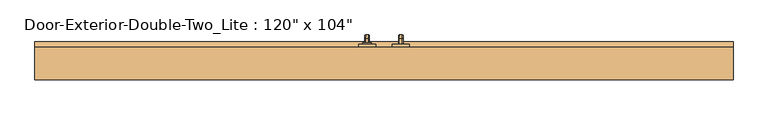
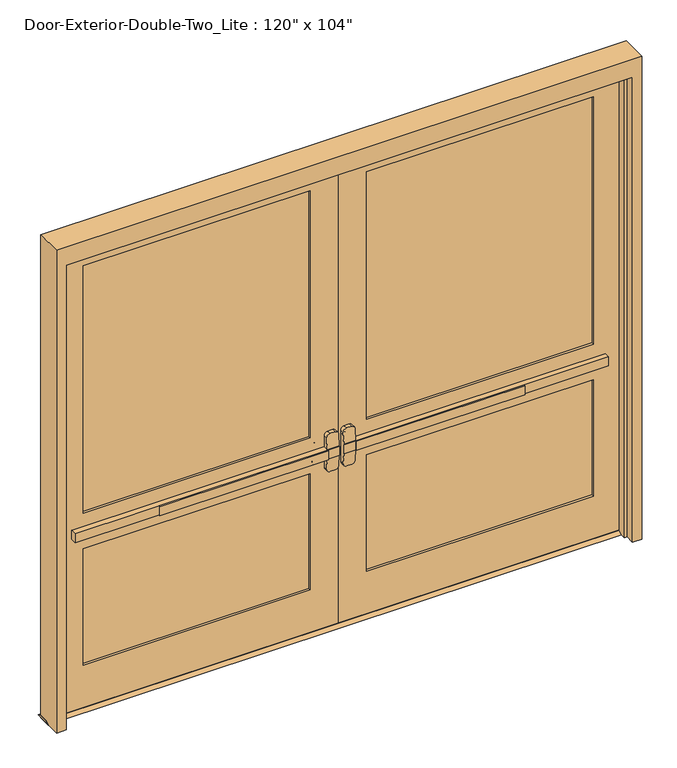
"""IFC4 building model written with IfcOpenShell, lengths in millimetres: door geometry."""

from ifc_helpers import new_model, si_unit, point, frame, frame_2d, origin, place, context, project, spatial, polyline, circle_curve, ellipse_curve, trimmed, segment, composite_curve, outline, extrude, faceted_brep, source, transform, mapped, element, save
from ifc_brep_helpers import plane_surface, cylinder_surface, revolved_surface, advanced_brep


def door_7b75190e(model_context):
    return source(origin(), model_context, "Body", "SolidModel", [
        extrude(outline(polyline([(-982.1333333, 0.0), (-982.1333333, 6.35), (-76.2, 6.35), (-76.2, 0.0), (-982.1333333, 0.0)])), frame((0.0, 0.0, 990.6), z_axis=(0.0, 0.0, 1.0), x_axis=(1.0, 0.0, 0.0)), (0.0, 0.0, 1.0), 50.8),
        advanced_brep(
        [(-12.7, 6.35, 1041.4), (-76.2, 6.35, 1041.4), (-1435.1, 6.35, 1041.4), (-1435.1, 6.35, 990.6), (-76.2, 6.35, 990.6), (-12.7, 6.35, 990.6), (-1435.1, 38.1, 1041.4), (-76.2, 38.1, 1041.4), (-76.2, 38.1, 1104.9), (-57.15, 38.1, 1123.95), (-31.75, 38.1, 1123.95), (-12.7, 38.1, 1104.9), (-12.7, 38.1, 927.1), (-31.75, 38.1, 908.05), (-57.15, 38.1, 908.05), (-76.2, 38.1, 927.1), (-76.2, 38.1, 990.6), (-1435.1, 38.1, 990.6), (-12.7, 9.5252467, 1041.4), (-76.2, 9.5252467, 1041.4), (-12.7, 9.5252467, 990.6), (-12.7, 14.5354269, 927.1), (-12.7, 14.5354269, 1104.9), (-76.2, 9.5252467, 990.6), (-76.2, 14.5354269, 1104.9), (-76.2, 14.5354269, 927.1), (-57.15, 16.038481, 1123.95), (-31.75, 16.038481, 1123.95), (-31.75, 16.038481, 908.05), (-57.15, 16.038481, 908.05)],
        [
            (0, 1),
            (1, 2),
            (2, 3),
            (3, 4),
            (4, 5),
            (5, 0),
            (6, 7),
            (7, 8),
            (8, 9, circle_curve(frame((-57.15, 38.1, 1104.9), z_axis=(0.0, 1.0, 0.0), x_axis=(-1.0, 0.0, 0.0)), 19.05)),
            (9, 10),
            (10, 11, circle_curve(frame((-31.75, 38.1, 1104.9), z_axis=(0.0, 1.0, 0.0), x_axis=(-1.0, 0.0, 0.0)), 19.05)),
            (11, 12),
            (12, 13, circle_curve(frame((-31.75, 38.1, 927.1), z_axis=(0.0, 1.0, 0.0), x_axis=(-1.0, 0.0, 0.0)), 19.05)),
            (13, 14),
            (14, 15, circle_curve(frame((-57.15, 38.1, 927.1), z_axis=(0.0, 1.0, 0.0), x_axis=(-1.0, 0.0, 0.0)), 19.05)),
            (15, 16),
            (16, 17),
            (17, 6),
            (0, 18),
            (18, 19),
            (19, 7),
            (6, 2),
            (5, 20),
            (20, 21),
            (21, 12),
            (11, 22),
            (22, 18),
            (16, 23),
            (23, 20),
            (3, 17),
            (19, 24),
            (24, 8),
            (15, 25),
            (25, 23),
            (9, 26),
            (26, 27),
            (27, 10),
            (13, 28),
            (28, 29),
            (29, 14),
            (29, 25, ellipse_curve(frame((-57.15, 14.5354269, 927.1), z_axis=(0.0, 0.9969018152893365, 0.07865602756830282), x_axis=(0.0, -0.07865602756830208, 0.9969018152893365)), 19.1092038, 19.05)),
            (24, 26, ellipse_curve(frame((-57.15, 14.5354269, 1104.9), z_axis=(0.0, 0.9969018152893376, -0.07865602756828934), x_axis=(0.0, -0.078656027568288, -0.9969018152893377)), 19.1092038, 19.05)),
            (27, 22, ellipse_curve(frame((-31.75, 14.5354269, 1104.9), z_axis=(0.0, 0.9969018152893376, -0.07865602756828934), x_axis=(0.0, -0.078656027568288, -0.9969018152893377)), 19.1092038, 19.05)),
            (21, 28, ellipse_curve(frame((-31.75, 14.5354269, 927.1), z_axis=(0.0, 0.9969018152893365, 0.07865602756830282), x_axis=(0.0, -0.07865602756830208, 0.9969018152893365)), 19.1092038, 19.05)),
        ],
        [
            plane_surface(frame((-12.7, 6.35, 1041.4), z_axis=(0.0, -1.0, 0.0), x_axis=(1.0, 0.0, 0.0))),
            plane_surface(frame((-12.7, 38.1, 1041.4), z_axis=(0.0, 1.0, 0.0), x_axis=(-1.0, 0.0, 0.0))),
            plane_surface(frame((-1435.1, 6.35, 1041.4), z_axis=(0.0, 0.0, 1.0), x_axis=(0.0, 1.0, 0.0))),
            plane_surface(frame((-12.7, 6.35, 1041.4), z_axis=(1.0, 0.0, 0.0), x_axis=(0.0, 1.0, 0.0))),
            plane_surface(frame((-12.7, 6.35, 990.6), z_axis=(0.0, 0.0, -1.0), x_axis=(0.0, 1.0, 0.0))),
            plane_surface(frame((-1435.1, 6.35, 990.6), z_axis=(-1.0, 0.0, 0.0), x_axis=(0.0, 1.0, 0.0))),
            plane_surface(frame((-76.2, 9.5252467, 927.1), z_axis=(-1.0, 0.0, 0.0), x_axis=(0.0, 1.0, 0.0))),
            plane_surface(frame((-57.15, 9.5252467, 1123.95), z_axis=(0.0, 0.0, 1.0), x_axis=(0.0, 1.0, 0.0))),
            plane_surface(frame((-31.75, 9.5252467, 908.05), z_axis=(0.0, 0.0, -1.0), x_axis=(0.0, 1.0, 0.0))),
            cylinder_surface(frame((-57.15, 38.1, 927.1), z_axis=(0.0, -1.0, 0.0), x_axis=(-1.0, 0.0, 0.0)), 19.05),
            cylinder_surface(frame((-57.15, 38.1, 1104.9), z_axis=(0.0, -1.0, 0.0), x_axis=(-1.0, 0.0, 0.0)), 19.05),
            cylinder_surface(frame((-31.75, 38.1, 1104.9), z_axis=(0.0, -1.0, 0.0), x_axis=(-1.0, 0.0, 0.0)), 19.05),
            cylinder_surface(frame((-31.75, 38.1, 927.1), z_axis=(0.0, -1.0, 0.0), x_axis=(-1.0, 0.0, 0.0)), 19.05),
            plane_surface(frame((-76.2, 9.5252467, 1041.4), z_axis=(0.0, -0.9969018152893376, 0.07865602756828934), x_axis=(1.0, 0.0, 0.0))),
            plane_surface(frame((-76.2, 16.038481, 908.05), z_axis=(0.0, -0.9969018152893365, -0.07865602756830282), x_axis=(1.0, 0.0, 0.0))),
        ],
        [
            (0, [[1, 2, 3, 4, 5, 6]]),
            (1, [[7, 8, 9, 10, 11, 12, 13, 14, 15, 16, 17, 18]]),
            (2, [[-2, -1, 19, 20, 21, -7, 22]]),
            (3, [[23, 24, 25, -12, 26, 27, -19, -6]]),
            (4, [[-17, 28, 29, -23, -5, -4, 30]]),
            (5, [[-22, -18, -30, -3]]),
            (6, [[-21, 31, 32, -8]]),
            (6, [[33, 34, -28, -16]]),
            (7, [[35, 36, 37, -10]]),
            (8, [[38, 39, 40, -14]]),
            (9, [[-40, 41, -33, -15]]),
            (10, [[-32, 42, -35, -9]]),
            (11, [[-37, 43, -26, -11]]),
            (12, [[-25, 44, -38, -13]]),
            (13, [[-27, -43, -36, -42, -31, -20]]),
            (14, [[-29, -34, -41, -39, -44, -24]]),
        ],
    ),
        extrude(outline(polyline([(82.55, 12.7), (107.95, 0.0), (12.7, 0.0), (38.1, 12.7), (82.55, 12.7)])), frame((-1574.8, 0.0, 0.0), z_axis=(1.0, 0.0, 0.0), x_axis=(0.0, 1.0, 0.0)), (0.0, 0.0, 1.0), 3149.6),
        extrude(outline(polyline([(982.1333333, 0.0), (76.2, 0.0), (76.2, 6.35), (982.1333333, 6.35), (982.1333333, 0.0)])), frame((0.0, 0.0, 990.6), z_axis=(0.0, 0.0, 1.0), x_axis=(1.0, 0.0, 0.0)), (0.0, 0.0, 1.0), 50.8),
        advanced_brep(
        [(12.7, 6.35, 1041.4), (12.7, 6.35, 990.6), (76.2, 6.35, 990.6), (1435.1, 6.35, 990.6), (1435.1, 6.35, 1041.4), (76.2, 6.35, 1041.4), (1435.1, 38.1, 1041.4), (1435.1, 38.1, 990.6), (76.2, 38.1, 990.6), (76.2, 38.1, 927.1), (57.15, 38.1, 908.05), (31.75, 38.1, 908.05), (12.7, 38.1, 927.1), (12.7, 38.1, 1104.9), (31.75, 38.1, 1123.95), (57.15, 38.1, 1123.95), (76.2, 38.1, 1104.9), (76.2, 38.1, 1041.4), (76.2, 9.5252467, 1041.4), (12.7, 9.5252467, 1041.4), (12.7, 14.5354269, 1104.9), (12.7, 14.5354269, 927.1), (12.7, 9.5252467, 990.6), (76.2, 9.5252467, 990.6), (76.2, 14.5354269, 927.1), (76.2, 14.5354269, 1104.9), (31.75, 16.038481, 1123.95), (57.15, 16.038481, 1123.95), (57.15, 16.038481, 908.05), (31.75, 16.038481, 908.05)],
        [
            (0, 1),
            (1, 2),
            (2, 3),
            (3, 4),
            (4, 5),
            (5, 0),
            (6, 7),
            (7, 8),
            (8, 9),
            (9, 10, circle_curve(frame((57.15, 38.1, 927.1), z_axis=(0.0, 1.0, 0.0), x_axis=(1.0, 0.0, 0.0)), 19.05)),
            (10, 11),
            (11, 12, circle_curve(frame((31.75, 38.1, 927.1), z_axis=(0.0, 1.0, 0.0), x_axis=(1.0, 0.0, 0.0)), 19.05)),
            (12, 13),
            (13, 14, circle_curve(frame((31.75, 38.1, 1104.9), z_axis=(0.0, 1.0, 0.0), x_axis=(1.0, 0.0, 0.0)), 19.05)),
            (14, 15),
            (15, 16, circle_curve(frame((57.15, 38.1, 1104.9), z_axis=(0.0, 1.0, 0.0), x_axis=(1.0, 0.0, 0.0)), 19.05)),
            (16, 17),
            (17, 6),
            (4, 6),
            (17, 18),
            (18, 19),
            (19, 0),
            (19, 20),
            (20, 13),
            (12, 21),
            (21, 22),
            (22, 1),
            (7, 3),
            (22, 23),
            (23, 8),
            (23, 24),
            (24, 9),
            (16, 25),
            (25, 18),
            (14, 26),
            (26, 27),
            (27, 15),
            (10, 28),
            (28, 29),
            (29, 11),
            (24, 28, ellipse_curve(frame((57.15, 14.5354269, 927.1), z_axis=(0.0, 0.9969018152893365, 0.07865602756830282), x_axis=(0.0, -0.07865602756830208, 0.9969018152893365)), 19.1092038, 19.05)),
            (27, 25, ellipse_curve(frame((57.15, 14.5354269, 1104.9), z_axis=(0.0, 0.9969018152893376, -0.07865602756828934), x_axis=(0.0, -0.078656027568288, -0.9969018152893377)), 19.1092038, 19.05)),
            (20, 26, ellipse_curve(frame((31.75, 14.5354269, 1104.9), z_axis=(0.0, 0.9969018152893376, -0.07865602756828934), x_axis=(0.0, -0.078656027568288, -0.9969018152893377)), 19.1092038, 19.05)),
            (29, 21, ellipse_curve(frame((31.75, 14.5354269, 927.1), z_axis=(0.0, 0.9969018152893365, 0.07865602756830282), x_axis=(0.0, -0.07865602756830208, 0.9969018152893365)), 19.1092038, 19.05)),
        ],
        [
            plane_surface(frame((12.7, 6.35, 1041.4), z_axis=(0.0, -1.0, 0.0), x_axis=(-1.0, 0.0, 0.0))),
            plane_surface(frame((12.7, 38.1, 1041.4), z_axis=(0.0, 1.0, 0.0), x_axis=(1.0, 0.0, 0.0))),
            plane_surface(frame((1435.1, 6.35, 1041.4), z_axis=(0.0, 0.0, 1.0), x_axis=(0.0, 1.0, 0.0))),
            plane_surface(frame((12.7, 6.35, 1041.4), z_axis=(-1.0, 0.0, 0.0), x_axis=(0.0, 1.0, 0.0))),
            plane_surface(frame((12.7, 6.35, 990.6), z_axis=(0.0, 0.0, -1.0), x_axis=(0.0, 1.0, 0.0))),
            plane_surface(frame((1435.1, 6.35, 990.6), z_axis=(1.0, 0.0, 0.0), x_axis=(0.0, 1.0, 0.0))),
            plane_surface(frame((76.2, 9.5252467, 927.1), z_axis=(1.0, 0.0, 0.0), x_axis=(0.0, 1.0, 0.0))),
            plane_surface(frame((57.15, 9.5252467, 1123.95), z_axis=(0.0, 0.0, 1.0), x_axis=(0.0, 1.0, 0.0))),
            plane_surface(frame((31.75, 9.5252467, 908.05), z_axis=(0.0, 0.0, -1.0), x_axis=(0.0, 1.0, 0.0))),
            cylinder_surface(frame((57.15, 38.1, 927.1), z_axis=(0.0, -1.0, 0.0), x_axis=(1.0, 0.0, 0.0)), 19.05),
            cylinder_surface(frame((57.15, 38.1, 1104.9), z_axis=(0.0, -1.0, 0.0), x_axis=(1.0, 0.0, 0.0)), 19.05),
            cylinder_surface(frame((31.75, 38.1, 1104.9), z_axis=(0.0, -1.0, 0.0), x_axis=(1.0, 0.0, 0.0)), 19.05),
            cylinder_surface(frame((31.75, 38.1, 927.1), z_axis=(0.0, -1.0, 0.0), x_axis=(1.0, 0.0, 0.0)), 19.05),
            plane_surface(frame((76.2, 9.5252467, 1041.4), z_axis=(0.0, -0.9969018152893376, 0.07865602756828934), x_axis=(-1.0, 0.0, 0.0))),
            plane_surface(frame((76.2, 16.038481, 908.05), z_axis=(0.0, -0.9969018152893365, -0.07865602756830282), x_axis=(-1.0, 0.0, 0.0))),
        ],
        [
            (0, [[1, 2, 3, 4, 5, 6]]),
            (1, [[7, 8, 9, 10, 11, 12, 13, 14, 15, 16, 17, 18]]),
            (2, [[19, -18, 20, 21, 22, -6, -5]]),
            (3, [[-1, -22, 23, 24, -13, 25, 26, 27]]),
            (4, [[28, -3, -2, -27, 29, 30, -8]]),
            (5, [[-4, -28, -7, -19]]),
            (6, [[-9, -30, 31, 32]]),
            (6, [[-17, 33, 34, -20]]),
            (7, [[-15, 35, 36, 37]]),
            (8, [[-11, 38, 39, 40]]),
            (9, [[-10, -32, 41, -38]]),
            (10, [[-16, -37, 42, -33]]),
            (11, [[-14, -24, 43, -35]]),
            (12, [[-12, -40, 44, -25]]),
            (13, [[-21, -34, -42, -36, -43, -23]]),
            (14, [[-26, -44, -39, -41, -31, -29]]),
        ],
    ),
        advanced_brep(
        [(66.2, 95.25, 1017.190625), (66.2, 95.25, 1014.809375), (69.771875, 95.25, 1011.2375), (82.6284594, 95.25, 1011.2375), (86.2, 95.25, 1014.8090406), (86.2, 95.25, 1017.190625), (82.628125, 95.25, 1020.7625), (69.771875, 95.25, 1020.7625), (66.2, 95.25, 887.809375), (69.771875, 95.25, 884.2375), (82.628125, 95.25, 884.2375), (86.2, 95.25, 887.809375), (86.2, 95.25, 890.1909594), (82.6284594, 95.25, 893.7625), (69.771875, 95.25, 893.7625), (66.2, 95.25, 890.190625), (66.2, 120.65, 1017.190625), (66.2, 134.540625, 1003.3), (66.2, 134.540625, 901.7), (66.2, 120.65, 887.809375), (66.2, 120.65, 890.190625), (66.2, 132.159375, 901.7), (66.2, 132.159375, 1003.3), (66.2, 120.65, 1014.809375), (69.771875, 120.65, 1011.2375), (82.6284594, 120.65, 1011.2375), (86.2, 120.65, 1014.8090406), (86.2, 132.1590406, 1003.3), (86.2, 132.1590406, 901.7), (86.2, 120.65, 890.1909594), (86.2, 120.65, 887.809375), (86.2, 134.540625, 901.7), (86.2, 134.540625, 1003.3), (86.2, 120.65, 1017.190625), (82.628125, 120.65, 1020.7625), (69.771875, 120.65, 1020.7625), (69.771875, 128.5875, 1003.3), (82.6284594, 128.5875, 1003.3), (82.628125, 138.1125, 1003.3), (69.771875, 138.1125, 1003.3), (69.771875, 128.5875, 901.7), (82.6284594, 128.5875, 901.7), (82.628125, 138.1125, 901.7), (69.771875, 138.1125, 901.7), (69.771875, 120.65, 893.7625), (82.6284594, 120.65, 893.7625), (82.628125, 120.65, 884.2375), (69.771875, 120.65, 884.2375)],
        [
            (0, 1),
            (1, 2, circle_curve(frame((69.771875, 95.25, 1014.809375), z_axis=(0.0, -1.0, 0.0), x_axis=(0.0, 0.0, 1.0)), 3.571875)),
            (2, 3),
            (3, 4, circle_curve(frame((82.6284594, 95.25, 1014.8090406), z_axis=(0.0, -1.0, 0.0), x_axis=(0.0, 0.0, 1.0)), 3.5715406)),
            (4, 5),
            (5, 6, circle_curve(frame((82.628125, 95.25, 1017.190625), z_axis=(0.0, -1.0, 0.0), x_axis=(0.0, 0.0, 1.0)), 3.571875)),
            (6, 7),
            (7, 0, circle_curve(frame((69.771875, 95.25, 1017.190625), z_axis=(0.0, -1.0, 0.0), x_axis=(0.0, 0.0, 1.0)), 3.571875)),
            (8, 9, circle_curve(frame((69.771875, 95.25, 887.809375), z_axis=(0.0, -1.0, 0.0), x_axis=(0.0, 0.0, -1.0)), 3.571875)),
            (9, 10),
            (10, 11, circle_curve(frame((82.628125, 95.25, 887.809375), z_axis=(0.0, -1.0, 0.0), x_axis=(0.0, 0.0, -1.0)), 3.571875)),
            (11, 12),
            (12, 13, circle_curve(frame((82.6284594, 95.25, 890.1909594), z_axis=(0.0, -1.0, 0.0), x_axis=(0.0, 0.0, -1.0)), 3.5715406)),
            (13, 14),
            (14, 15, circle_curve(frame((69.771875, 95.25, 890.190625), z_axis=(0.0, -1.0, 0.0), x_axis=(0.0, 0.0, -1.0)), 3.571875)),
            (15, 8),
            (0, 16),
            (16, 17, circle_curve(frame((66.2, 120.65, 1003.3), z_axis=(-1.0, 0.0, 0.0), x_axis=(0.0, 0.0, 1.0)), 13.890625)),
            (17, 18),
            (18, 19, circle_curve(frame((66.2, 120.65, 901.7), z_axis=(-1.0, 0.0, 0.0), x_axis=(0.0, 1.0, 0.0)), 13.890625)),
            (19, 8),
            (15, 20),
            (20, 21, circle_curve(frame((66.2, 120.65, 901.7), z_axis=(1.0, 0.0, 0.0), x_axis=(0.0, 1.0, 0.0)), 11.509375)),
            (21, 22),
            (22, 23, circle_curve(frame((66.2, 120.65, 1003.3), z_axis=(1.0, 0.0, 0.0), x_axis=(0.0, 0.0, 1.0)), 11.509375)),
            (23, 1),
            (23, 24, circle_curve(frame((69.771875, 120.65, 1014.809375), z_axis=(0.0, -1.0, 0.0), x_axis=(0.0, 0.0, 1.0)), 3.571875)),
            (24, 2),
            (24, 25),
            (25, 3),
            (25, 26, circle_curve(frame((82.6284594, 120.65, 1014.8090406), z_axis=(0.0, -1.0, 0.0), x_axis=(0.0, 0.0, 1.0)), 3.5715406)),
            (26, 4),
            (26, 27, circle_curve(frame((86.2, 120.65, 1003.3), z_axis=(-1.0, 0.0, 0.0), x_axis=(0.0, 0.0, 1.0)), 11.5090406)),
            (27, 28),
            (28, 29, circle_curve(frame((86.2, 120.65, 901.7), z_axis=(-1.0, 0.0, 0.0), x_axis=(0.0, 1.0, 0.0)), 11.5090406)),
            (29, 12),
            (11, 30),
            (30, 31, circle_curve(frame((86.2, 120.65, 901.7), z_axis=(1.0, 0.0, 0.0), x_axis=(0.0, 1.0, 0.0)), 13.890625)),
            (31, 32),
            (32, 33, circle_curve(frame((86.2, 120.65, 1003.3), z_axis=(1.0, 0.0, 0.0), x_axis=(0.0, 0.0, 1.0)), 13.890625)),
            (33, 5),
            (33, 34, circle_curve(frame((82.628125, 120.65, 1017.190625), z_axis=(0.0, -1.0, 0.0), x_axis=(0.0, 0.0, 1.0)), 3.571875)),
            (34, 6),
            (34, 35),
            (35, 7),
            (35, 16, circle_curve(frame((69.771875, 120.65, 1017.190625), z_axis=(0.0, -1.0, 0.0), x_axis=(0.0, 0.0, 1.0)), 3.571875)),
            (36, 24, circle_curve(frame((69.771875, 120.65, 1003.3), z_axis=(1.0, 0.0, 0.0), x_axis=(0.0, 0.0, 1.0)), 7.9375)),
            (22, 36, circle_curve(frame((69.771875, 132.159375, 1003.3), z_axis=(0.0, 0.0, 1.0), x_axis=(0.0, 1.0, 0.0)), 3.571875)),
            (37, 25, circle_curve(frame((82.6284594, 120.65, 1003.3), z_axis=(1.0, 0.0, 0.0), x_axis=(0.0, 0.0, 1.0)), 7.9375)),
            (36, 37),
            (37, 27, circle_curve(frame((82.6284594, 132.1590406, 1003.3), z_axis=(0.0, 0.0, 1.0), x_axis=(0.0, 1.0, 0.0)), 3.5715406)),
            (38, 34, circle_curve(frame((82.628125, 120.65, 1003.3), z_axis=(1.0, 0.0, 0.0), x_axis=(0.0, 0.0, 1.0)), 17.4625)),
            (32, 38, circle_curve(frame((82.628125, 134.540625, 1003.3), z_axis=(0.0, 0.0, 1.0), x_axis=(0.0, 1.0, 0.0)), 3.571875)),
            (39, 35, circle_curve(frame((69.771875, 120.65, 1003.3), z_axis=(1.0, 0.0, 0.0), x_axis=(0.0, 0.0, 1.0)), 17.4625)),
            (38, 39),
            (39, 17, circle_curve(frame((69.771875, 134.540625, 1003.3), z_axis=(0.0, 0.0, 1.0), x_axis=(0.0, 1.0, 0.0)), 3.571875)),
            (21, 40, circle_curve(frame((69.771875, 132.159375, 901.7), z_axis=(0.0, 0.0, 1.0), x_axis=(0.0, 1.0, 0.0)), 3.571875)),
            (40, 36),
            (40, 41),
            (41, 37),
            (41, 28, circle_curve(frame((82.6284594, 132.1590406, 901.7), z_axis=(0.0, 0.0, 1.0), x_axis=(0.0, 1.0, 0.0)), 3.5715406)),
            (31, 42, circle_curve(frame((82.628125, 134.540625, 901.7), z_axis=(0.0, 0.0, 1.0), x_axis=(0.0, 1.0, 0.0)), 3.571875)),
            (42, 38),
            (42, 43),
            (43, 39),
            (43, 18, circle_curve(frame((69.771875, 134.540625, 901.7), z_axis=(0.0, 0.0, 1.0), x_axis=(0.0, 1.0, 0.0)), 3.571875)),
            (44, 40, circle_curve(frame((69.771875, 120.65, 901.7), z_axis=(1.0, 0.0, 0.0), x_axis=(0.0, 1.0, 0.0)), 7.9375)),
            (20, 44, circle_curve(frame((69.771875, 120.65, 890.190625), z_axis=(0.0, 1.0, 0.0), x_axis=(0.0, 0.0, -1.0)), 3.571875)),
            (45, 41, circle_curve(frame((82.6284594, 120.65, 901.7), z_axis=(1.0, 0.0, 0.0), x_axis=(0.0, 1.0, 0.0)), 7.9375)),
            (44, 45),
            (45, 29, circle_curve(frame((82.6284594, 120.65, 890.1909594), z_axis=(0.0, 1.0, 0.0), x_axis=(0.0, 0.0, -1.0)), 3.5715406)),
            (46, 42, circle_curve(frame((82.628125, 120.65, 901.7), z_axis=(1.0, 0.0, 0.0), x_axis=(0.0, 1.0, 0.0)), 17.4625)),
            (30, 46, circle_curve(frame((82.628125, 120.65, 887.809375), z_axis=(0.0, 1.0, 0.0), x_axis=(0.0, 0.0, -1.0)), 3.571875)),
            (47, 43, circle_curve(frame((69.771875, 120.65, 901.7), z_axis=(1.0, 0.0, 0.0), x_axis=(0.0, 1.0, 0.0)), 17.4625)),
            (46, 47),
            (47, 19, circle_curve(frame((69.771875, 120.65, 887.809375), z_axis=(0.0, 1.0, 0.0), x_axis=(0.0, 0.0, -1.0)), 3.571875)),
            (14, 44),
            (13, 45),
            (10, 46),
            (9, 47),
        ],
        [
            plane_surface(frame((76.2, 95.25, 1016.0), z_axis=(0.0, -1.0, 0.0), x_axis=(1.0, 0.0, 0.0))),
            plane_surface(frame((76.2, 95.25, 889.0), z_axis=(0.0, -1.0, 0.0), x_axis=(1.0, 0.0, 0.0))),
            plane_surface(frame((66.2, 95.25, 1017.190625), z_axis=(-1.0, 0.0, 0.0), x_axis=(0.0, 1.0, 0.0))),
            cylinder_surface(frame((69.771875, 95.25, 1014.809375), z_axis=(0.0, -1.0, 0.0), x_axis=(0.0, 0.0, 1.0)), 3.571875),
            plane_surface(frame((69.771875, 95.25, 1011.2375), z_axis=(0.0, 0.0, -1.0), x_axis=(0.0, 1.0, 0.0))),
            cylinder_surface(frame((82.6284594, 95.25, 1014.8090406), z_axis=(0.0, -1.0, 0.0), x_axis=(0.0, 0.0, 1.0)), 3.5715406),
            plane_surface(frame((86.2, 95.25, 1014.8090406), z_axis=(1.0, 0.0, 0.0), x_axis=(0.0, 1.0, 0.0))),
            cylinder_surface(frame((82.628125, 95.25, 1017.190625), z_axis=(0.0, -1.0, 0.0), x_axis=(0.0, 0.0, 1.0)), 3.571875),
            plane_surface(frame((82.628125, 95.25, 1020.7625), z_axis=(0.0, 0.0, 1.0), x_axis=(0.0, 1.0, 0.0))),
            cylinder_surface(frame((69.771875, 95.25, 1017.190625), z_axis=(0.0, -1.0, 0.0), x_axis=(0.0, 0.0, 1.0)), 3.571875),
            revolved_surface(trimmed(ellipse_curve(frame((69.771875, 120.65, 1014.809375), z_axis=(0.0, -1.0, 0.0), x_axis=(0.0, 0.0, 1.0)), 3.571875, 3.571875), [point((66.2, 120.65, 1014.809375))], [point((69.771875, 120.65, 1011.2375))], True, "CARTESIAN"), (76.2, 120.65, 1003.3), (-1.0, 0.0, 0.0)),
            revolved_surface(polyline([(69.771875, 120.65, 1011.2375), (82.6284594, 120.65, 1011.2375)]), (76.2, 120.65, 1003.3), (-1.0, 0.0, 0.0)),
            revolved_surface(trimmed(ellipse_curve(frame((82.6284594, 120.65, 1014.8090406), z_axis=(0.0, -1.0, 0.0), x_axis=(0.0, 0.0, 1.0)), 3.5715406, 3.5715406), [point((82.6284594, 120.65, 1011.2375))], [point((86.2, 120.65, 1014.8090406))], True, "CARTESIAN"), (76.2, 120.65, 1003.3), (-1.0, 0.0, 0.0)),
            revolved_surface(trimmed(ellipse_curve(frame((82.628125, 120.65, 1017.190625), z_axis=(0.0, -1.0, 0.0), x_axis=(0.0, 0.0, 1.0)), 3.571875, 3.571875), [point((86.2, 120.65, 1017.190625))], [point((82.628125, 120.65, 1020.7625))], True, "CARTESIAN"), (76.2, 120.65, 1003.3), (-1.0, 0.0, 0.0)),
            cylinder_surface(frame((76.2, 120.65, 1003.3), z_axis=(-1.0, 0.0, 0.0), x_axis=(0.0, 0.0, 1.0)), 17.4625),
            revolved_surface(trimmed(ellipse_curve(frame((69.771875, 120.65, 1017.190625), z_axis=(0.0, -1.0, 0.0), x_axis=(0.0, 0.0, 1.0)), 3.571875, 3.571875), [point((69.771875, 120.65, 1020.7625))], [point((66.2, 120.65, 1017.190625))], True, "CARTESIAN"), (76.2, 120.65, 1003.3), (-1.0, 0.0, 0.0)),
            cylinder_surface(frame((69.771875, 132.159375, 1003.3), z_axis=(0.0, 0.0, 1.0), x_axis=(0.0, 1.0, 0.0)), 3.571875),
            plane_surface(frame((69.771875, 128.5875, 1003.3), z_axis=(0.0, -1.0, 0.0), x_axis=(0.0, 0.0, -1.0))),
            cylinder_surface(frame((82.6284594, 132.1590406, 1003.3), z_axis=(0.0, 0.0, 1.0), x_axis=(0.0, 1.0, 0.0)), 3.5715406),
            cylinder_surface(frame((82.628125, 134.540625, 1003.3), z_axis=(0.0, 0.0, 1.0), x_axis=(0.0, 1.0, 0.0)), 3.571875),
            plane_surface(frame((82.628125, 138.1125, 1003.3), z_axis=(0.0, 1.0, 0.0), x_axis=(0.0, 0.0, -1.0))),
            cylinder_surface(frame((69.771875, 134.540625, 1003.3), z_axis=(0.0, 0.0, 1.0), x_axis=(0.0, 1.0, 0.0)), 3.571875),
            revolved_surface(trimmed(ellipse_curve(frame((69.771875, 132.159375, 901.7), z_axis=(0.0, 0.0, 1.0), x_axis=(0.0, 1.0, 0.0)), 3.571875, 3.571875), [point((66.2, 132.159375, 901.7))], [point((69.771875, 128.5875, 901.7))], True, "CARTESIAN"), (76.2, 120.65, 901.7), (-1.0, 0.0, 0.0)),
            revolved_surface(polyline([(69.771875, 128.5875, 901.7), (82.6284594, 128.5875, 901.7)]), (76.2, 120.65, 901.7), (-1.0, 0.0, 0.0)),
            revolved_surface(trimmed(ellipse_curve(frame((82.6284594, 132.1590406, 901.7), z_axis=(0.0, 0.0, 1.0), x_axis=(0.0, 1.0, 0.0)), 3.5715406, 3.5715406), [point((82.6284594, 128.5875, 901.7))], [point((86.2, 132.1590406, 901.7))], True, "CARTESIAN"), (76.2, 120.65, 901.7), (-1.0, 0.0, 0.0)),
            revolved_surface(trimmed(ellipse_curve(frame((82.628125, 134.540625, 901.7), z_axis=(0.0, 0.0, 1.0), x_axis=(0.0, 1.0, 0.0)), 3.571875, 3.571875), [point((86.2, 134.540625, 901.7))], [point((82.628125, 138.1125, 901.7))], True, "CARTESIAN"), (76.2, 120.65, 901.7), (-1.0, 0.0, 0.0)),
            cylinder_surface(frame((76.2, 120.65, 901.7), z_axis=(-1.0, 0.0, 0.0), x_axis=(0.0, 1.0, 0.0)), 17.4625),
            revolved_surface(trimmed(ellipse_curve(frame((69.771875, 134.540625, 901.7), z_axis=(0.0, 0.0, 1.0), x_axis=(0.0, 1.0, 0.0)), 3.571875, 3.571875), [point((69.771875, 138.1125, 901.7))], [point((66.2, 134.540625, 901.7))], True, "CARTESIAN"), (76.2, 120.65, 901.7), (-1.0, 0.0, 0.0)),
            cylinder_surface(frame((69.771875, 120.65, 890.190625), z_axis=(0.0, 1.0, 0.0), x_axis=(0.0, 0.0, -1.0)), 3.571875),
            plane_surface(frame((69.771875, 120.65, 893.7625), z_axis=(0.0, 0.0, 1.0), x_axis=(0.0, -1.0, 0.0))),
            cylinder_surface(frame((82.6284594, 120.65, 890.1909594), z_axis=(0.0, 1.0, 0.0), x_axis=(0.0, 0.0, -1.0)), 3.5715406),
            cylinder_surface(frame((82.628125, 120.65, 887.809375), z_axis=(0.0, 1.0, 0.0), x_axis=(0.0, 0.0, -1.0)), 3.571875),
            plane_surface(frame((82.628125, 120.65, 884.2375), z_axis=(0.0, 0.0, -1.0), x_axis=(0.0, -1.0, 0.0))),
            cylinder_surface(frame((69.771875, 120.65, 887.809375), z_axis=(0.0, 1.0, 0.0), x_axis=(0.0, 0.0, -1.0)), 3.571875),
        ],
        [
            (0, [[1, 2, 3, 4, 5, 6, 7, 8]]),
            (1, [[9, 10, 11, 12, 13, 14, 15, 16]]),
            (2, [[-1, 17, 18, 19, 20, 21, -16, 22, 23, 24, 25, 26]]),
            (3, [[-2, -26, 27, 28]]),
            (4, [[-3, -28, 29, 30]]),
            (5, [[-4, -30, 31, 32]]),
            (6, [[-5, -32, 33, 34, 35, 36, -12, 37, 38, 39, 40, 41]]),
            (7, [[-6, -41, 42, 43]]),
            (8, [[-7, -43, 44, 45]]),
            (9, [[-8, -45, 46, -17]]),
            (10, [[47, -27, -25, 48]]),
            (11, [[49, -29, -47, 50]]),
            (12, [[-33, -31, -49, 51]]),
            (13, [[52, -42, -40, 53]]),
            (14, [[54, -44, -52, 55]]),
            (15, [[-18, -46, -54, 56]]),
            (16, [[-48, -24, 57, 58]]),
            (17, [[-50, -58, 59, 60]]),
            (18, [[-51, -60, 61, -34]]),
            (19, [[-53, -39, 62, 63]]),
            (20, [[-55, -63, 64, 65]]),
            (21, [[-56, -65, 66, -19]]),
            (22, [[67, -57, -23, 68]]),
            (23, [[69, -59, -67, 70]]),
            (24, [[-35, -61, -69, 71]]),
            (25, [[72, -62, -38, 73]]),
            (26, [[74, -64, -72, 75]]),
            (27, [[-20, -66, -74, 76]]),
            (28, [[-68, -22, -15, 77]]),
            (29, [[-70, -77, -14, 78]]),
            (30, [[-71, -78, -13, -36]]),
            (31, [[-73, -37, -11, 79]]),
            (32, [[-75, -79, -10, 80]]),
            (33, [[-76, -80, -9, -21]]),
        ],
    ),
        extrude(outline(composite_curve([segment(trimmed(circle_curve(frame_2d((1113.0338574, 76.2)), 89.3016225), [point((1193.8, 114.3))], [point((1193.8, 38.1))], False, "CARTESIAN"), True, "CONTINUOUS"), segment(polyline([(1193.8, 38.1), (838.2, 38.1)]), True, "CONTINUOUS"), segment(trimmed(circle_curve(frame_2d((918.9661426, 76.2)), 89.3016225), [point((838.2, 38.1))], [point((838.2, 114.3))], False, "CARTESIAN"), True, "CONTINUOUS"), segment(polyline([(838.2, 114.3), (1193.8, 114.3)]), True, "CONTINUOUS")], self_intersect=False)), frame((0.0, 82.55, 0.0), z_axis=(0.0, 1.0, 0.0), x_axis=(0.0, 0.0, 1.0)), (0.0, 0.0, 1.0), 12.7),
        advanced_brep(
        [(-86.2, 95.25, 1017.190625), (-86.2, 95.25, 1014.809375), (-82.628125, 95.25, 1011.2375), (-69.7715406, 95.25, 1011.2375), (-66.2, 95.25, 1014.8090406), (-66.2, 95.25, 1017.190625), (-69.771875, 95.25, 1020.7625), (-82.628125, 95.25, 1020.7625), (-86.2, 95.25, 887.809375), (-82.628125, 95.25, 884.2375), (-69.771875, 95.25, 884.2375), (-66.2, 95.25, 887.809375), (-66.2, 95.25, 890.1909594), (-69.7715406, 95.25, 893.7625), (-82.628125, 95.25, 893.7625), (-86.2, 95.25, 890.190625), (-86.2, 120.65, 1017.190625), (-86.2, 134.540625, 1003.3), (-86.2, 134.540625, 901.7), (-86.2, 120.65, 887.809375), (-86.2, 120.65, 890.190625), (-86.2, 132.159375, 901.7), (-86.2, 132.159375, 1003.3), (-86.2, 120.65, 1014.809375), (-82.628125, 120.65, 1011.2375), (-69.7715406, 120.65, 1011.2375), (-66.2, 120.65, 1014.8090406), (-66.2, 132.1590406, 1003.3), (-66.2, 132.1590406, 901.7), (-66.2, 120.65, 890.1909594), (-66.2, 120.65, 887.809375), (-66.2, 134.540625, 901.7), (-66.2, 134.540625, 1003.3), (-66.2, 120.65, 1017.190625), (-69.771875, 120.65, 1020.7625), (-82.628125, 120.65, 1020.7625), (-82.628125, 128.5875, 1003.3), (-69.7715406, 128.5875, 1003.3), (-69.771875, 138.1125, 1003.3), (-82.628125, 138.1125, 1003.3), (-82.628125, 128.5875, 901.7), (-69.7715406, 128.5875, 901.7), (-69.771875, 138.1125, 901.7), (-82.628125, 138.1125, 901.7), (-82.628125, 120.65, 893.7625), (-69.7715406, 120.65, 893.7625), (-69.771875, 120.65, 884.2375), (-82.628125, 120.65, 884.2375)],
        [
            (0, 1),
            (1, 2, circle_curve(frame((-82.628125, 95.25, 1014.809375), z_axis=(0.0, -1.0, 0.0), x_axis=(0.0, 0.0, 1.0)), 3.571875)),
            (2, 3),
            (3, 4, circle_curve(frame((-69.7715406, 95.25, 1014.8090406), z_axis=(0.0, -1.0, 0.0), x_axis=(0.0, 0.0, 1.0)), 3.5715406)),
            (4, 5),
            (5, 6, circle_curve(frame((-69.771875, 95.25, 1017.190625), z_axis=(0.0, -1.0, 0.0), x_axis=(0.0, 0.0, 1.0)), 3.571875)),
            (6, 7),
            (7, 0, circle_curve(frame((-82.628125, 95.25, 1017.190625), z_axis=(0.0, -1.0, 0.0), x_axis=(0.0, 0.0, 1.0)), 3.571875)),
            (8, 9, circle_curve(frame((-82.628125, 95.25, 887.809375), z_axis=(0.0, -1.0, 0.0), x_axis=(0.0, 0.0, -1.0)), 3.571875)),
            (9, 10),
            (10, 11, circle_curve(frame((-69.771875, 95.25, 887.809375), z_axis=(0.0, -1.0, 0.0), x_axis=(0.0, 0.0, -1.0)), 3.571875)),
            (11, 12),
            (12, 13, circle_curve(frame((-69.7715406, 95.25, 890.1909594), z_axis=(0.0, -1.0, 0.0), x_axis=(0.0, 0.0, -1.0)), 3.5715406)),
            (13, 14),
            (14, 15, circle_curve(frame((-82.628125, 95.25, 890.190625), z_axis=(0.0, -1.0, 0.0), x_axis=(0.0, 0.0, -1.0)), 3.571875)),
            (15, 8),
            (0, 16),
            (16, 17, circle_curve(frame((-86.2, 120.65, 1003.3), z_axis=(-1.0, 0.0, 0.0), x_axis=(0.0, 0.0, 1.0)), 13.890625)),
            (17, 18),
            (18, 19, circle_curve(frame((-86.2, 120.65, 901.7), z_axis=(-1.0, 0.0, 0.0), x_axis=(0.0, 1.0, 0.0)), 13.890625)),
            (19, 8),
            (15, 20),
            (20, 21, circle_curve(frame((-86.2, 120.65, 901.7), z_axis=(1.0, 0.0, 0.0), x_axis=(0.0, 1.0, 0.0)), 11.509375)),
            (21, 22),
            (22, 23, circle_curve(frame((-86.2, 120.65, 1003.3), z_axis=(1.0, 0.0, 0.0), x_axis=(0.0, 0.0, 1.0)), 11.509375)),
            (23, 1),
            (23, 24, circle_curve(frame((-82.628125, 120.65, 1014.809375), z_axis=(0.0, -1.0, 0.0), x_axis=(0.0, 0.0, 1.0)), 3.571875)),
            (24, 2),
            (24, 25),
            (25, 3),
            (25, 26, circle_curve(frame((-69.7715406, 120.65, 1014.8090406), z_axis=(0.0, -1.0, 0.0), x_axis=(0.0, 0.0, 1.0)), 3.5715406)),
            (26, 4),
            (26, 27, circle_curve(frame((-66.2, 120.65, 1003.3), z_axis=(-1.0, 0.0, 0.0), x_axis=(0.0, 0.0, 1.0)), 11.5090406)),
            (27, 28),
            (28, 29, circle_curve(frame((-66.2, 120.65, 901.7), z_axis=(-1.0, 0.0, 0.0), x_axis=(0.0, 1.0, 0.0)), 11.5090406)),
            (29, 12),
            (11, 30),
            (30, 31, circle_curve(frame((-66.2, 120.65, 901.7), z_axis=(1.0, 0.0, 0.0), x_axis=(0.0, 1.0, 0.0)), 13.890625)),
            (31, 32),
            (32, 33, circle_curve(frame((-66.2, 120.65, 1003.3), z_axis=(1.0, 0.0, 0.0), x_axis=(0.0, 0.0, 1.0)), 13.890625)),
            (33, 5),
            (33, 34, circle_curve(frame((-69.771875, 120.65, 1017.190625), z_axis=(0.0, -1.0, 0.0), x_axis=(0.0, 0.0, 1.0)), 3.571875)),
            (34, 6),
            (34, 35),
            (35, 7),
            (35, 16, circle_curve(frame((-82.628125, 120.65, 1017.190625), z_axis=(0.0, -1.0, 0.0), x_axis=(0.0, 0.0, 1.0)), 3.571875)),
            (36, 24, circle_curve(frame((-82.628125, 120.65, 1003.3), z_axis=(1.0, 0.0, 0.0), x_axis=(0.0, 0.0, 1.0)), 7.9375)),
            (22, 36, circle_curve(frame((-82.628125, 132.159375, 1003.3), z_axis=(0.0, 0.0, 1.0), x_axis=(0.0, 1.0, 0.0)), 3.571875)),
            (37, 25, circle_curve(frame((-69.7715406, 120.65, 1003.3), z_axis=(1.0, 0.0, 0.0), x_axis=(0.0, 0.0, 1.0)), 7.9375)),
            (36, 37),
            (37, 27, circle_curve(frame((-69.7715406, 132.1590406, 1003.3), z_axis=(0.0, 0.0, 1.0), x_axis=(0.0, 1.0, 0.0)), 3.5715406)),
            (38, 34, circle_curve(frame((-69.771875, 120.65, 1003.3), z_axis=(1.0, 0.0, 0.0), x_axis=(0.0, 0.0, 1.0)), 17.4625)),
            (32, 38, circle_curve(frame((-69.771875, 134.540625, 1003.3), z_axis=(0.0, 0.0, 1.0), x_axis=(0.0, 1.0, 0.0)), 3.571875)),
            (39, 35, circle_curve(frame((-82.628125, 120.65, 1003.3), z_axis=(1.0, 0.0, 0.0), x_axis=(0.0, 0.0, 1.0)), 17.4625)),
            (38, 39),
            (39, 17, circle_curve(frame((-82.628125, 134.540625, 1003.3), z_axis=(0.0, 0.0, 1.0), x_axis=(0.0, 1.0, 0.0)), 3.571875)),
            (21, 40, circle_curve(frame((-82.628125, 132.159375, 901.7), z_axis=(0.0, 0.0, 1.0), x_axis=(0.0, 1.0, 0.0)), 3.571875)),
            (40, 36),
            (40, 41),
            (41, 37),
            (41, 28, circle_curve(frame((-69.7715406, 132.1590406, 901.7), z_axis=(0.0, 0.0, 1.0), x_axis=(0.0, 1.0, 0.0)), 3.5715406)),
            (31, 42, circle_curve(frame((-69.771875, 134.540625, 901.7), z_axis=(0.0, 0.0, 1.0), x_axis=(0.0, 1.0, 0.0)), 3.571875)),
            (42, 38),
            (42, 43),
            (43, 39),
            (43, 18, circle_curve(frame((-82.628125, 134.540625, 901.7), z_axis=(0.0, 0.0, 1.0), x_axis=(0.0, 1.0, 0.0)), 3.571875)),
            (44, 40, circle_curve(frame((-82.628125, 120.65, 901.7), z_axis=(1.0, 0.0, 0.0), x_axis=(0.0, 1.0, 0.0)), 7.9375)),
            (20, 44, circle_curve(frame((-82.628125, 120.65, 890.190625), z_axis=(0.0, 1.0, 0.0), x_axis=(0.0, 0.0, -1.0)), 3.571875)),
            (45, 41, circle_curve(frame((-69.7715406, 120.65, 901.7), z_axis=(1.0, 0.0, 0.0), x_axis=(0.0, 1.0, 0.0)), 7.9375)),
            (44, 45),
            (45, 29, circle_curve(frame((-69.7715406, 120.65, 890.1909594), z_axis=(0.0, 1.0, 0.0), x_axis=(0.0, 0.0, -1.0)), 3.5715406)),
            (46, 42, circle_curve(frame((-69.771875, 120.65, 901.7), z_axis=(1.0, 0.0, 0.0), x_axis=(0.0, 1.0, 0.0)), 17.4625)),
            (30, 46, circle_curve(frame((-69.771875, 120.65, 887.809375), z_axis=(0.0, 1.0, 0.0), x_axis=(0.0, 0.0, -1.0)), 3.571875)),
            (47, 43, circle_curve(frame((-82.628125, 120.65, 901.7), z_axis=(1.0, 0.0, 0.0), x_axis=(0.0, 1.0, 0.0)), 17.4625)),
            (46, 47),
            (47, 19, circle_curve(frame((-82.628125, 120.65, 887.809375), z_axis=(0.0, 1.0, 0.0), x_axis=(0.0, 0.0, -1.0)), 3.571875)),
            (14, 44),
            (13, 45),
            (10, 46),
            (9, 47),
        ],
        [
            plane_surface(frame((-76.2, 95.25, 1016.0), z_axis=(0.0, -1.0, 0.0), x_axis=(1.0, 0.0, 0.0))),
            plane_surface(frame((-76.2, 95.25, 889.0), z_axis=(0.0, -1.0, 0.0), x_axis=(1.0, 0.0, 0.0))),
            plane_surface(frame((-86.2, 95.25, 1017.190625), z_axis=(-1.0, 0.0, 0.0), x_axis=(0.0, 1.0, 0.0))),
            cylinder_surface(frame((-82.628125, 95.25, 1014.809375), z_axis=(0.0, -1.0, 0.0), x_axis=(0.0, 0.0, 1.0)), 3.571875),
            plane_surface(frame((-82.628125, 95.25, 1011.2375), z_axis=(0.0, 0.0, -1.0), x_axis=(0.0, 1.0, 0.0))),
            cylinder_surface(frame((-69.7715406, 95.25, 1014.8090406), z_axis=(0.0, -1.0, 0.0), x_axis=(0.0, 0.0, 1.0)), 3.5715406),
            plane_surface(frame((-66.2, 95.25, 1014.8090406), z_axis=(1.0, 0.0, 0.0), x_axis=(0.0, 1.0, 0.0))),
            cylinder_surface(frame((-69.771875, 95.25, 1017.190625), z_axis=(0.0, -1.0, 0.0), x_axis=(0.0, 0.0, 1.0)), 3.571875),
            plane_surface(frame((-69.771875, 95.25, 1020.7625), z_axis=(0.0, 0.0, 1.0), x_axis=(0.0, 1.0, 0.0))),
            cylinder_surface(frame((-82.628125, 95.25, 1017.190625), z_axis=(0.0, -1.0, 0.0), x_axis=(0.0, 0.0, 1.0)), 3.571875),
            revolved_surface(trimmed(ellipse_curve(frame((-82.628125, 120.65, 1014.809375), z_axis=(0.0, -1.0, 0.0), x_axis=(0.0, 0.0, 1.0)), 3.571875, 3.571875), [point((-86.2, 120.65, 1014.809375))], [point((-82.628125, 120.65, 1011.2375))], True, "CARTESIAN"), (-76.2, 120.65, 1003.3), (-1.0, 0.0, 0.0)),
            revolved_surface(polyline([(-82.628125, 120.65, 1011.2375), (-69.7715406, 120.65, 1011.2375)]), (-76.2, 120.65, 1003.3), (-1.0, 0.0, 0.0)),
            revolved_surface(trimmed(ellipse_curve(frame((-69.7715406, 120.65, 1014.8090406), z_axis=(0.0, -1.0, 0.0), x_axis=(0.0, 0.0, 1.0)), 3.5715406, 3.5715406), [point((-69.7715406, 120.65, 1011.2375))], [point((-66.2, 120.65, 1014.8090406))], True, "CARTESIAN"), (-76.2, 120.65, 1003.3), (-1.0, 0.0, 0.0)),
            revolved_surface(trimmed(ellipse_curve(frame((-69.771875, 120.65, 1017.190625), z_axis=(0.0, -1.0, 0.0), x_axis=(0.0, 0.0, 1.0)), 3.571875, 3.571875), [point((-66.2, 120.65, 1017.190625))], [point((-69.771875, 120.65, 1020.7625))], True, "CARTESIAN"), (-76.2, 120.65, 1003.3), (-1.0, 0.0, 0.0)),
            cylinder_surface(frame((-76.2, 120.65, 1003.3), z_axis=(-1.0, 0.0, 0.0), x_axis=(0.0, 0.0, 1.0)), 17.4625),
            revolved_surface(trimmed(ellipse_curve(frame((-82.628125, 120.65, 1017.190625), z_axis=(0.0, -1.0, 0.0), x_axis=(0.0, 0.0, 1.0)), 3.571875, 3.571875), [point((-82.628125, 120.65, 1020.7625))], [point((-86.2, 120.65, 1017.190625))], True, "CARTESIAN"), (-76.2, 120.65, 1003.3), (-1.0, 0.0, 0.0)),
            cylinder_surface(frame((-82.628125, 132.159375, 1003.3), z_axis=(0.0, 0.0, 1.0), x_axis=(0.0, 1.0, 0.0)), 3.571875),
            plane_surface(frame((-82.628125, 128.5875, 1003.3), z_axis=(0.0, -1.0, 0.0), x_axis=(0.0, 0.0, -1.0))),
            cylinder_surface(frame((-69.7715406, 132.1590406, 1003.3), z_axis=(0.0, 0.0, 1.0), x_axis=(0.0, 1.0, 0.0)), 3.5715406),
            cylinder_surface(frame((-69.771875, 134.540625, 1003.3), z_axis=(0.0, 0.0, 1.0), x_axis=(0.0, 1.0, 0.0)), 3.571875),
            plane_surface(frame((-69.771875, 138.1125, 1003.3), z_axis=(0.0, 1.0, 0.0), x_axis=(0.0, 0.0, -1.0))),
            cylinder_surface(frame((-82.628125, 134.540625, 1003.3), z_axis=(0.0, 0.0, 1.0), x_axis=(0.0, 1.0, 0.0)), 3.571875),
            revolved_surface(trimmed(ellipse_curve(frame((-82.628125, 132.159375, 901.7), z_axis=(0.0, 0.0, 1.0), x_axis=(0.0, 1.0, 0.0)), 3.571875, 3.571875), [point((-86.2, 132.159375, 901.7))], [point((-82.628125, 128.5875, 901.7))], True, "CARTESIAN"), (-76.2, 120.65, 901.7), (-1.0, 0.0, 0.0)),
            revolved_surface(polyline([(-82.628125, 128.5875, 901.7), (-69.7715406, 128.5875, 901.7)]), (-76.2, 120.65, 901.7), (-1.0, 0.0, 0.0)),
            revolved_surface(trimmed(ellipse_curve(frame((-69.7715406, 132.1590406, 901.7), z_axis=(0.0, 0.0, 1.0), x_axis=(0.0, 1.0, 0.0)), 3.5715406, 3.5715406), [point((-69.7715406, 128.5875, 901.7))], [point((-66.2, 132.1590406, 901.7))], True, "CARTESIAN"), (-76.2, 120.65, 901.7), (-1.0, 0.0, 0.0)),
            revolved_surface(trimmed(ellipse_curve(frame((-69.771875, 134.540625, 901.7), z_axis=(0.0, 0.0, 1.0), x_axis=(0.0, 1.0, 0.0)), 3.571875, 3.571875), [point((-66.2, 134.540625, 901.7))], [point((-69.771875, 138.1125, 901.7))], True, "CARTESIAN"), (-76.2, 120.65, 901.7), (-1.0, 0.0, 0.0)),
            cylinder_surface(frame((-76.2, 120.65, 901.7), z_axis=(-1.0, 0.0, 0.0), x_axis=(0.0, 1.0, 0.0)), 17.4625),
            revolved_surface(trimmed(ellipse_curve(frame((-82.628125, 134.540625, 901.7), z_axis=(0.0, 0.0, 1.0), x_axis=(0.0, 1.0, 0.0)), 3.571875, 3.571875), [point((-82.628125, 138.1125, 901.7))], [point((-86.2, 134.540625, 901.7))], True, "CARTESIAN"), (-76.2, 120.65, 901.7), (-1.0, 0.0, 0.0)),
            cylinder_surface(frame((-82.628125, 120.65, 890.190625), z_axis=(0.0, 1.0, 0.0), x_axis=(0.0, 0.0, -1.0)), 3.571875),
            plane_surface(frame((-82.628125, 120.65, 893.7625), z_axis=(0.0, 0.0, 1.0), x_axis=(0.0, -1.0, 0.0))),
            cylinder_surface(frame((-69.7715406, 120.65, 890.1909594), z_axis=(0.0, 1.0, 0.0), x_axis=(0.0, 0.0, -1.0)), 3.5715406),
            cylinder_surface(frame((-69.771875, 120.65, 887.809375), z_axis=(0.0, 1.0, 0.0), x_axis=(0.0, 0.0, -1.0)), 3.571875),
            plane_surface(frame((-69.771875, 120.65, 884.2375), z_axis=(0.0, 0.0, -1.0), x_axis=(0.0, -1.0, 0.0))),
            cylinder_surface(frame((-82.628125, 120.65, 887.809375), z_axis=(0.0, 1.0, 0.0), x_axis=(0.0, 0.0, -1.0)), 3.571875),
        ],
        [
            (0, [[1, 2, 3, 4, 5, 6, 7, 8]]),
            (1, [[9, 10, 11, 12, 13, 14, 15, 16]]),
            (2, [[-1, 17, 18, 19, 20, 21, -16, 22, 23, 24, 25, 26]]),
            (3, [[-2, -26, 27, 28]]),
            (4, [[-3, -28, 29, 30]]),
            (5, [[-4, -30, 31, 32]]),
            (6, [[-5, -32, 33, 34, 35, 36, -12, 37, 38, 39, 40, 41]]),
            (7, [[-6, -41, 42, 43]]),
            (8, [[-7, -43, 44, 45]]),
            (9, [[-8, -45, 46, -17]]),
            (10, [[47, -27, -25, 48]]),
            (11, [[49, -29, -47, 50]]),
            (12, [[-33, -31, -49, 51]]),
            (13, [[52, -42, -40, 53]]),
            (14, [[54, -44, -52, 55]]),
            (15, [[-18, -46, -54, 56]]),
            (16, [[-48, -24, 57, 58]]),
            (17, [[-50, -58, 59, 60]]),
            (18, [[-51, -60, 61, -34]]),
            (19, [[-53, -39, 62, 63]]),
            (20, [[-55, -63, 64, 65]]),
            (21, [[-56, -65, 66, -19]]),
            (22, [[67, -57, -23, 68]]),
            (23, [[69, -59, -67, 70]]),
            (24, [[-35, -61, -69, 71]]),
            (25, [[72, -62, -38, 73]]),
            (26, [[74, -64, -72, 75]]),
            (27, [[-20, -66, -74, 76]]),
            (28, [[-68, -22, -15, 77]]),
            (29, [[-70, -77, -14, 78]]),
            (30, [[-71, -78, -13, -36]]),
            (31, [[-73, -37, -11, 79]]),
            (32, [[-75, -79, -10, 80]]),
            (33, [[-76, -80, -9, -21]]),
        ],
    ),
        extrude(outline(composite_curve([segment(trimmed(circle_curve(frame_2d((1117.6, -76.2)), 19.0), [point((1117.6, -95.2))], [point((1117.6, -57.2))], False, "CARTESIAN"), True, "CONTINUOUS"), segment(trimmed(circle_curve(frame_2d((1117.6, -76.2)), 19.0), [point((1117.6, -57.2))], [point((1117.6, -95.2))], False, "CARTESIAN"), True, "CONTINUOUS")], self_intersect=False)), frame((0.0, 95.25, 0.0), z_axis=(0.0, 1.0, 0.0), x_axis=(0.0, 0.0, 1.0)), (0.0, 0.0, 1.0), 8.73125),
        extrude(outline(composite_curve([segment(trimmed(circle_curve(frame_2d((1113.0338574, -76.2)), 89.3016225), [point((1193.8, -38.1))], [point((1193.8, -114.3))], False, "CARTESIAN"), True, "CONTINUOUS"), segment(polyline([(1193.8, -114.3), (838.2, -114.3)]), True, "CONTINUOUS"), segment(trimmed(circle_curve(frame_2d((918.9661426, -76.2)), 89.3016225), [point((838.2, -114.3))], [point((838.2, -38.1))], False, "CARTESIAN"), True, "CONTINUOUS"), segment(polyline([(838.2, -38.1), (1193.8, -38.1)]), True, "CONTINUOUS")], self_intersect=False)), frame((0.0, 82.55, 0.0), z_axis=(0.0, 1.0, 0.0), x_axis=(0.0, 0.0, 1.0)), (0.0, 0.0, 1.0), 12.7),
        faceted_brep([(1524.0, 33.3375, 0.0), (1524.0, 82.55, 0.0), (1574.8, 82.55, 0.0), (1574.8, -63.5, 0.0), (1524.0, -63.5, 0.0), (1524.0, -14.2875, 0.0), (1508.125, -14.2875, 0.0), (1508.125, 33.3375, 0.0), (1524.0, 33.3375, 2641.6), (1524.0, 82.55, 2641.6), (-1524.0, 82.55, 2641.6), (-1524.0, 82.55, 0.0), (-1574.8, 82.55, 0.0), (-1574.8, 82.55, 2743.2), (1574.8, 82.55, 2743.2), (1574.8, -63.5, 2743.2), (-1574.8, -63.5, 2743.2), (-1574.8, -63.5, 0.0), (-1524.0, -63.5, 0.0), (-1524.0, -63.5, 2641.6), (1524.0, -63.5, 2641.6), (1524.0, -14.2875, 2641.6), (-1524.0, -14.2875, 2641.6), (-1524.0, -14.2875, 0.0), (-1508.125, -14.2875, 0.0), (-1508.125, -14.2875, 2625.725), (1508.125, -14.2875, 2625.725), (1508.125, 33.3375, 2625.725), (-1508.125, 33.3375, 2625.725), (-1508.125, 33.3375, 0.0), (-1524.0, 33.3375, 0.0), (-1524.0, 33.3375, 2641.6)], [[[0, 1, 2, 3, 4, 5, 6, 7]], [[1, 0, 8, 9]], [[2, 1, 9, 10, 11, 12, 13, 14]], [[3, 2, 14, 15]], [[4, 3, 15, 16, 17, 18, 19, 20]], [[5, 4, 20, 21]], [[6, 5, 21, 22, 23, 24, 25, 26]], [[7, 6, 26, 27]], [[0, 7, 27, 28, 29, 30, 31, 8]], [[9, 8, 31, 10]], [[20, 19, 22, 21]], [[26, 25, 28, 27]], [[12, 11, 30, 29, 24, 23, 18, 17]], [[11, 10, 31, 30]], [[13, 12, 17, 16]], [[19, 18, 23, 22]], [[25, 24, 29, 28]], [[15, 14, 13, 16]]]),
        extrude(outline(polyline([(2641.6, 1.5875), (12.7, 1.5875), (12.7, 1524.0), (2641.6, 1524.0), (2641.6, 1.5875)]), holes=[polyline([(2524.125, 152.4), (2524.125, 1371.6), (1117.6, 1371.6), (1117.6, 152.4), (2524.125, 152.4)]), polyline([(914.4, 152.4), (914.4, 1371.6), (254.0, 1371.6), (254.0, 152.4), (914.4, 152.4)])]), frame((0.0, 38.1, 0.0), z_axis=(0.0, 1.0, 0.0), x_axis=(0.0, 0.0, 1.0)), (0.0, 0.0, 1.0), 44.45),
        extrude(outline(polyline([(12.7, -1.5875), (2641.6, -1.5875), (2641.6, -1524.0), (12.7, -1524.0), (12.7, -1.5875)]), holes=[polyline([(2524.125, -1371.6), (2524.125, -152.4), (1117.6, -152.4), (1117.6, -1371.6), (2524.125, -1371.6)]), polyline([(914.4, -1371.6), (914.4, -152.4), (254.0, -152.4), (254.0, -1371.6), (914.4, -1371.6)])]), frame((0.0, 38.1, 0.0), z_axis=(0.0, 1.0, 0.0), x_axis=(0.0, 0.0, 1.0)), (0.0, 0.0, 1.0), 44.45),
        extrude(outline(polyline([(1371.6, 50.8), (152.4, 50.8), (152.4, 69.85), (1371.6, 69.85), (1371.6, 50.8)])), frame((0.0, 0.0, 1117.6), z_axis=(0.0, 0.0, 1.0), x_axis=(1.0, 0.0, 0.0)), (0.0, 0.0, 1.0), 1406.525),
        extrude(outline(polyline([(-152.4, 50.8), (-1371.6, 50.8), (-1371.6, 69.85), (-152.4, 69.85), (-152.4, 50.8)])), frame((0.0, 0.0, 1117.6), z_axis=(0.0, 0.0, 1.0), x_axis=(1.0, 0.0, 0.0)), (0.0, 0.0, 1.0), 1406.525),
        extrude(outline(polyline([(-152.4, 50.8), (-1371.6, 50.8), (-1371.6, 69.85), (-152.4, 69.85), (-152.4, 50.8)])), frame((0.0, 0.0, 254.0), z_axis=(0.0, 0.0, 1.0), x_axis=(1.0, 0.0, 0.0)), (0.0, 0.0, 1.0), 660.4),
        extrude(outline(polyline([(1371.6, 50.8), (152.4, 50.8), (152.4, 69.85), (1371.6, 69.85), (1371.6, 50.8)])), frame((0.0, 0.0, 254.0), z_axis=(0.0, 0.0, 1.0), x_axis=(1.0, 0.0, 0.0)), (0.0, 0.0, 1.0), 660.4),
    ])


if __name__ == "__main__":
    model = new_model("IFC4")
    model_context = context("Model", 3, world=origin())
    ifc_project = project(units=[si_unit("LENGTHUNIT", "METRE", prefix="MILLI")], contexts=[model_context])
    site = spatial("IfcSite", under=ifc_project)
    building = spatial("IfcBuilding", under=site)
    placement = place(None, origin())
    door_shape = door_7b75190e(model_context)
    element("IfcDoor", 1, ObjectType="Door-Exterior-Double-Two_Lite : 120\" x 104\"", at=placement, inside=building, context=model_context, shape_type="MappedRepresentation", body=[
        mapped(door_shape, transform((0.0, 0.0, 0.0), x_axis=(1.0, 0.0, 0.0), y_axis=(0.0, 1.0, 0.0), z_axis=(0.0, 0.0, 1.0))),
    ])
    save(model, "model.ifc")

# Revit data of these elements
# Type "Door-Exterior-Double-Two_Lite : 120\" x 104\""
#   Type Mark = "10"
#   Assembly Code = "B2030100"
#   Analytic Construction = "Metal frame, double glass door"
#   Top Rail = 0' - 4 5/8"
#   Threshold Length [instance default] = 10' - 4"
#   Threshold Offset [instance default] = 0' - 0 1/2"
#   Thickness = 0' - 1 3/4"
#   Thermal Resistance (R) = 1.3794 (h·ft²·°F)/BTU
#   Swing Angle [instance default] = 90.00°
#   Strike Height = 3' - 4"
#   Stiles = 0' - 6"
#   SinglePanelWidth = 5' - 0"
#   Rough Width [instance default] = 10' - 4"
#   Rough Height [instance default] = 9' - 0"
#   MFOpeningHeight [instance default] = 0' - 4"
#   MFOpeningWidth [instance default] = 0' - 4"
#   Lock Rail = 0' - 8"
#   Inset Calculate [instance default] = 0' - 4"
#   Masonry Inset [instance default] = 0' - 1"
#   Height = 8' - 8"
#   Width = 10' - 0"
#   Heat Transfer Coefficient (U) = 0.7250 BTU/(h·ft²·°F)
#   Glass Thickness = 0' - 0 3/4"
#   Masonry Frame Depth = 0' - 5 3/4"
#   Bottom Rail = 0' - 10"
#   Threshold [instance default] = yes
#   Masonry Frame [instance default] = yes
#   Function = 1
#   Dry Wall Frame [instance default] = no
#   Threshold Material = none
#   Panic Bar Material = Metal - Stainless Steel
#   Panel Material = Metal - Painted - Grey
#   Glass Stop Material = Metal - Painted - Grey
#   Frame Material = Metal - Painted - Grey
#   Exterior Pull Material = Metal - Stainless Steel
#   Visual Light Transmittance = 0
#   Solar Heat Gain Coefficient = 0
#   Wall Closure = (empty or 0)
# Element 1 (IfcDoor, "Door-Exterior-Double-Two_Lite : 120\" x 104\"")
#   Materials on its faces: "Metal - Painted - Grey", "Metal - Stainless Steel", "Glass"
# Materials
#   "Metal - Stainless Steel": class "Metal", colour RGB 247 247 247, transparency 0
#   "Metal - Painted - Grey": class "Paint", colour RGB 104 104 104, transparency 0, Cost = 0
#   "Glass": class "Glass", colour RGB 0 128 192, transparency 0.75, Description = "Soda Lime Glass", Cost = 0
